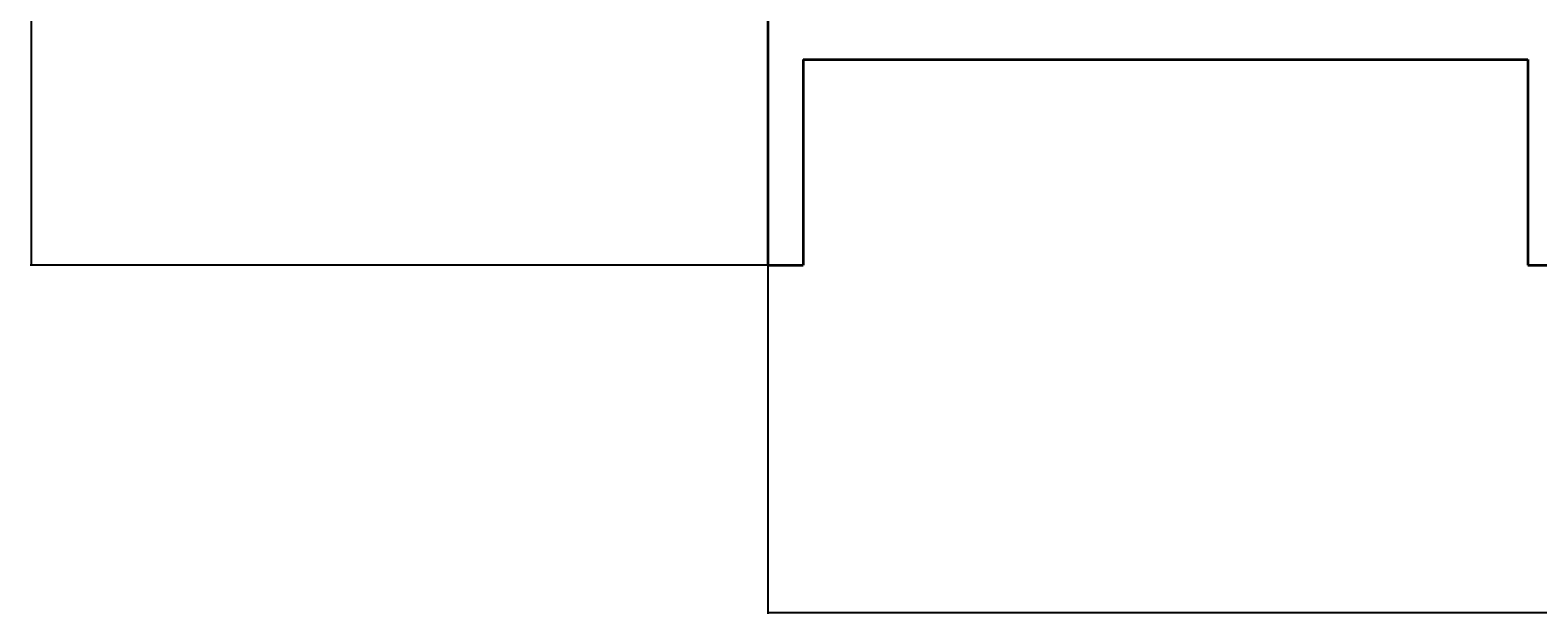
# Model space of a CAD drawing. Units: inches. Extents: x 3731 to 4318, y 1310 to 2388.
# Tile 1 of 57: x 3731 to 3944, y 1310 to 1393. Entities that reach past the tile are written whole.
import ezdxf

# ---------------------------------------------------------------- set-up
doc = ezdxf.new("R2010")
doc.units = ezdxf.units.IN
doc.layers.add('A-ANNO-DIMS', color=2, linetype='Continuous', lineweight=18)
doc.layers.add('A-WALL', color=7, linetype='Continuous', lineweight=35)
doc.styles.get("Standard").update_dxf_attribs({"font": 'arial.ttf'})
doc.dimstyles.get("Standard").update_dxf_attribs({"dimtxt": 0.18, "dimasz": 0.18, "dimexe": 0.18, "dimexo": 0.0625, "dimgap": 0.09, "dimtad": 0, "dimtih": 1, "dimtoh": 1, "dimdec": 4, "dimzin": 0, "dimdsep": 46, "dimtxsty": 'Standard', "dimcen": 0.09, "dimadec": 0, "dimazin": 0, "dimtfac": 1, "dimtdec": 4, "dimtofl": 0, "dimtmove": 0, "dimatfit": 3, "dimfxl": 1, "dimtolj": 1, "dimtzin": 0, "dimarcsym": 0})

# ---------------------------------------------------------------- blocks, each defined once
blk = doc.blocks.new('*D32')
at = {"layer": 'A-ANNO-DIMS', "color": 0, "lineweight": -2, "transparency": 16777216}
for p, q in [((4269.21, 1592.32), (4269.21, 1310.25)), ((3835.21, 1359.32), (3835.21, 1310.25)), ((3835.39, 1310.43), (4051.92, 1310.43)), ((4269.03, 1310.43), (4052.5, 1310.43))]:
    blk.add_line(p, q, dxfattribs=at)
at = {"layer": 'A-ANNO-DIMS', "color": 0, "transparency": 16777216}
for points in [[(3835.39, 1310.46), (3835.39, 1310.4), (3835.21, 1310.43)], [(4269.03, 1310.46), (4269.03, 1310.4), (4269.21, 1310.43)]]:
    blk.add_solid(points, dxfattribs=at)
at = {"layer": 'Defpoints', "color": 0, "transparency": 16777216}
for p in [(4269.21, 1592.38), (3835.21, 1359.38), (4269.21, 1310.43)]:
    blk.add_point(p, dxfattribs=at)
at = {"layer": 'A-ANNO-DIMS', "color": 0, "transparency": 16777216, "insert": (4052.21, 1310.43), "char_height": 0.18, "attachment_point": 5}
blk.add_mtext('\\A1;434', dxfattribs=at)
blk = doc.blocks.new('*D33')
at = {"layer": 'A-ANNO-DIMS', "color": 0, "lineweight": -2, "transparency": 16777216}
for p, q in [((3835.15, 2338.38), (3731.41, 2338.38)), ((3731.59, 2338.2), (3731.59, 1849.06)), ((3731.59, 1359.56), (3731.59, 1848.7)), ((3835.15, 1359.38), (3731.41, 1359.38))]:
    blk.add_line(p, q, dxfattribs=at)
at = {"layer": 'A-ANNO-DIMS', "color": 0, "transparency": 16777216}
for points in [[(3731.56, 2338.2), (3731.62, 2338.2), (3731.59, 2338.38)], [(3731.56, 1359.56), (3731.62, 1359.56), (3731.59, 1359.38)]]:
    blk.add_solid(points, dxfattribs=at)
at = {"layer": 'Defpoints', "color": 0, "transparency": 16777216}
for p in [(3731.59, 2338.38), (3835.21, 2338.38), (3835.21, 1359.38)]:
    blk.add_point(p, dxfattribs=at)
at = {"layer": 'A-ANNO-DIMS', "color": 0, "transparency": 16777216, "insert": (3731.59, 1848.88), "char_height": 0.18, "attachment_point": 5}
blk.add_mtext('\\A1;979', dxfattribs=at)

msp = doc.modelspace()

# ---------------------------------------------------------------- linework, layer by layer
at = {"layer": 'A-WALL'}
for p, q in [((3835.21, 2338.38), (3835.21, 1359.38)), ((3840.21, 1388.38), (3942.21, 1388.38)), ((3840.21, 1388.38), (3840.21, 1359.38)), ((3942.21, 1388.38), (3942.21, 1359.38)), ((3835.21, 1359.38), (3840.21, 1359.38)), ((3942.21, 1359.38), (4239.21, 1359.38))]:
    msp.add_line(p, q, dxfattribs=at)

# ---------------------------------------------------------------- dimensions: what is measured, and where the dimension line sits
at = {"layer": 'A-ANNO-DIMS'}
dim = msp.add_linear_dim(base=(3731.59, 2338.38), p1=(3835.21, 1359.38), p2=(3835.21, 2338.38), angle=90, dimstyle='Standard', override={"dimdec": 0, "dimlfac": 1, "dimrnd": 0, "dimzin": 0, "dimdsep": 46, "dimlunit": 2}, dxfattribs=at)
dim.commit()
dim.dimension.update_dxf_attribs({"geometry": '*D33', "text_midpoint": (3731.59, 1848.88)})
dim = msp.add_linear_dim(base=(4269.21, 1310.43), p1=(3835.21, 1359.38), p2=(4269.21, 1592.38), dimstyle='Standard', override={"dimdec": 0, "dimlfac": 1, "dimrnd": 0, "dimzin": 0, "dimdsep": 46, "dimlunit": 2}, dxfattribs=at)
dim.commit()
dim.dimension.update_dxf_attribs({"geometry": '*D32', "text_midpoint": (4052.21, 1310.43)})

doc.saveas('drawing.dxf')
